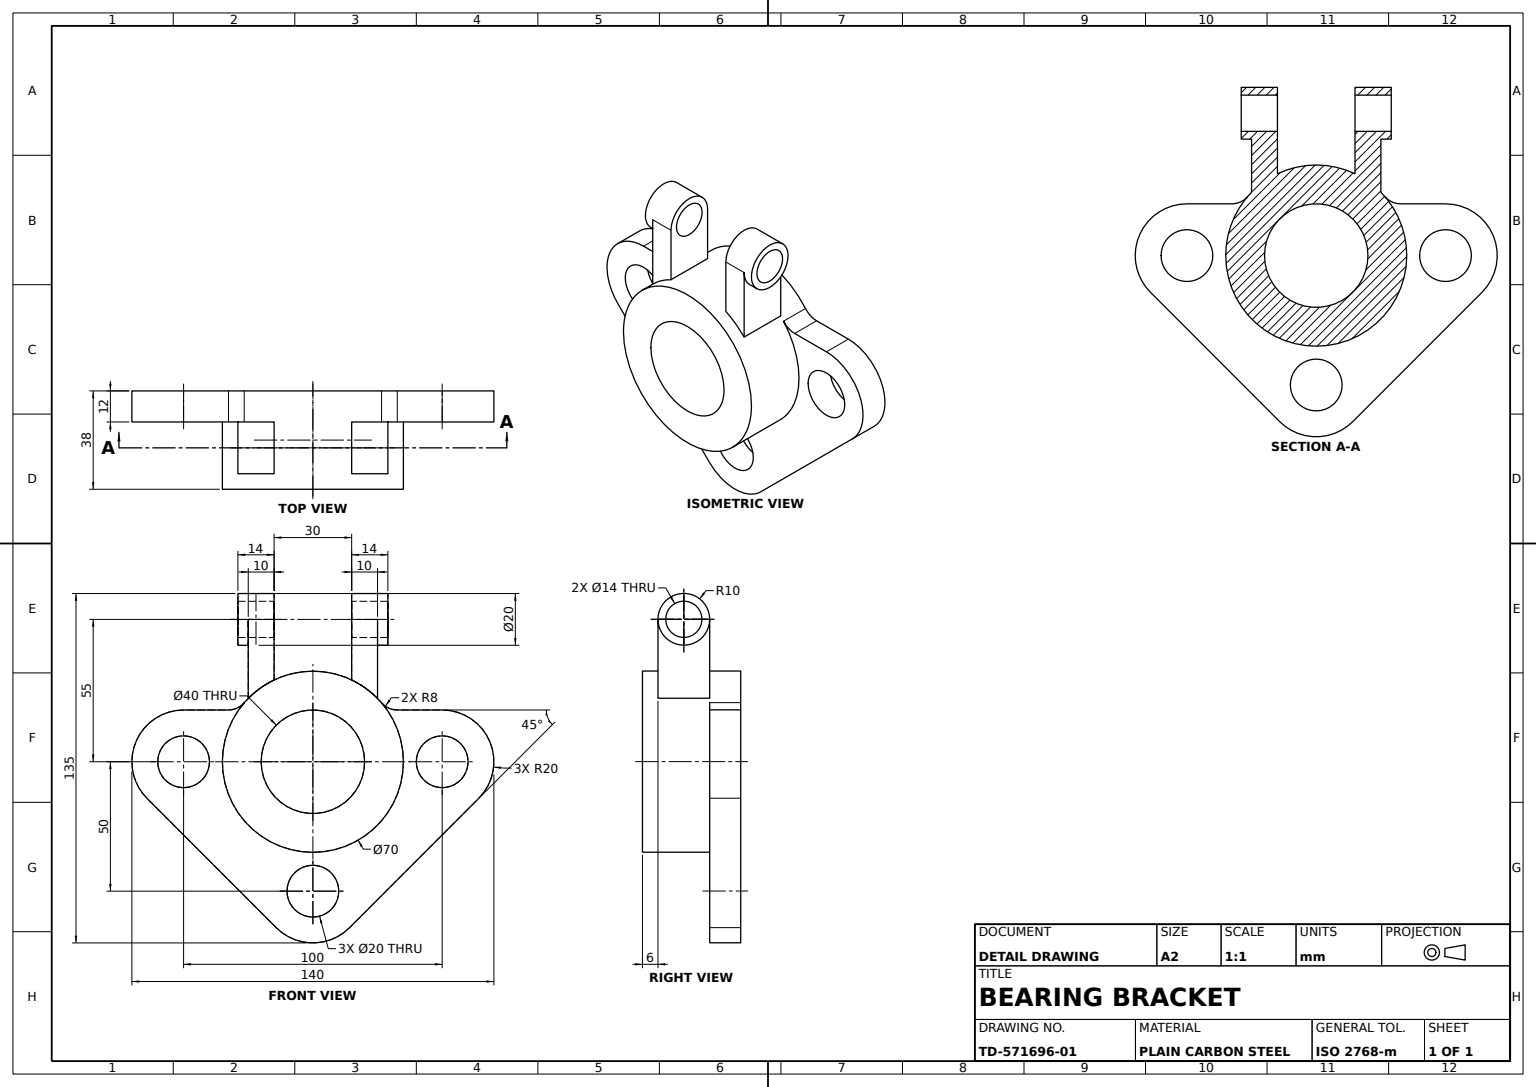
SolidWorks part; units mm, degrees
material "Plain Carbon Steel"
ref_plane "Front Plane" through (0, 0, 0) normal (0, 0, 1) x (1, 0, 0)
ref_plane "Top Plane" through (0, 0, 0) normal (0, 1, 0) x (1, 0, 0)
ref_plane "Right Plane" through (0, 0, 0) normal (1, 0, 0) x (0, 0, -1)
sketch "Hub Profile Sketch" plane through (0, 0, 0) normal (0, 0, 1) x (1, 0, 0)
  circle A0 centre (0, 0) radius 35
  circle A1 centre (0, 0) radius 20
  dimension "D1" = 70
  dimension "D2" = 40
extrude "Hub Ø70 Bore Ø40" add sketch "Hub Profile Sketch" along normal blind 38
ref_plane "Plane1" through (0, 0, 0) normal (0, 0, 1) x (1, 0, 0)
sketch "Mounting Flange Sketch" plane through (0, 0, 0) normal (0, 0, 1) x (1, 0, 0)
  line L0 (50, 20) -> (28.7228, 20)
  line L2 (-64.1421, -14.1421) -> (-14.1421, -64.1421)
  line L3 (14.1421, -64.1421) -> (64.1421, -14.1421)
  line L4 (-50, 20) -> (-28.7228, 20)
  circle A0 centre (50, 0) radius 10
  arc A1 (64.1421, -14.1421) -> (50, 20) centre (50, 0) ccw
  circle A2 centre (0, -50) radius 10
  arc A3 (-14.1421, -64.1421) -> (14.1421, -64.1421) centre (0, -50) ccw
  circle A4 centre (0, 0) radius 35 construction
  circle A5 centre (-50, 0) radius 10
  arc A6 (-64.1421, -14.1421) -> (-50, 20) centre (-50, 0) cw
  arc A7 (-28.7228, 20) -> (28.7228, 20) centre (0, 0) ccw
  dimension "D1" = 40
  dimension "D2" = 20
  dimension "D4" = 50
  dimension "D5" = 40
  dimension "D6" = 20
  dimension "D9" = 35
  dimension "D10" = 20
  dimension "D3" = 50
  dimension "D7" = 100
  dimension "D8" = 50
extrude "Mounting Flange" add sketch "Mounting Flange Sketch" along normal blind 12
fillet "Flange Hub Fillet R8" radius 8 2 edges at (-28.7228, 20, 6) (28.7228, 20, 6)
ref_plane "Plane2" through (0, 55, 0) normal (0, 1, 0) x (1, 0, 0)
sketch "Clevis Lug Sketch" plane through (0, 55, 0) normal (0, 1, 0) x (1, 0, 0)
  line L0 (-32.6343, -12) -> (-26.5628, -12) construction
  line L1 (-15, -32) -> (-25, -32)
  line L2 (-15, -32) -> (-15, -12)
  line L3 (-15, -12) -> (-25, -12)
  line L4 (-25, -32) -> (-25, -12)
  line L5 (0, 0) -> (0, -38) construction
  line L6 (-35, -38) -> (35, -38) construction
  line L7 (15, -32) -> (25, -32)
  line L8 (15, -32) -> (15, -12)
  line L9 (15, -12) -> (25, -12)
  line L10 (25, -32) -> (25, -12)
  dimension "D1" = 6
  dimension "D2" = 10
  dimension "D3" = 30
extrude "Clevis Lugs" add sketch "Clevis Lug Sketch" against normal blind 32
sketch "Lug Boss Sketch A" plane through (15, 0, 0) normal (-1, 0, 0) x (0, 0, 1)
  line L0 (12, 55) -> (32, 55) construction
  circle A0 centre (22, 55) radius 10
  circle A1 centre (22, 55) radius 7
  dimension "D1" = 14
  dimension "D2" = 20
extrude "Lug Boss A Ø20" add sketch "Lug Boss Sketch A" against normal blind 14
sketch "Pin Hole Sketch" plane through (25, 0, 0) normal (1, 0, 0) x (0, 0, -1)
  line L0 (-29, 55) -> (-15, 55) construction
  circle A0 centre (-22, 55) radius 7
  dimension "D1" = 14
extrude "Pin Hole Ø14" cut sketch "Pin Hole Sketch" against normal blind 50
sketch "Lug Boss Sketch B" plane through (-15, 0, 0) normal (1, 0, 0) x (0, 0, -1)
  circle A0 centre (-22, 55) radius 7
  circle A1 centre (-22, 55) radius 10
  dimension "D1" = 20
  dimension "D2" = 14
extrude "Lug Boss B Ø20" add sketch "Lug Boss Sketch B" against normal blind 14
